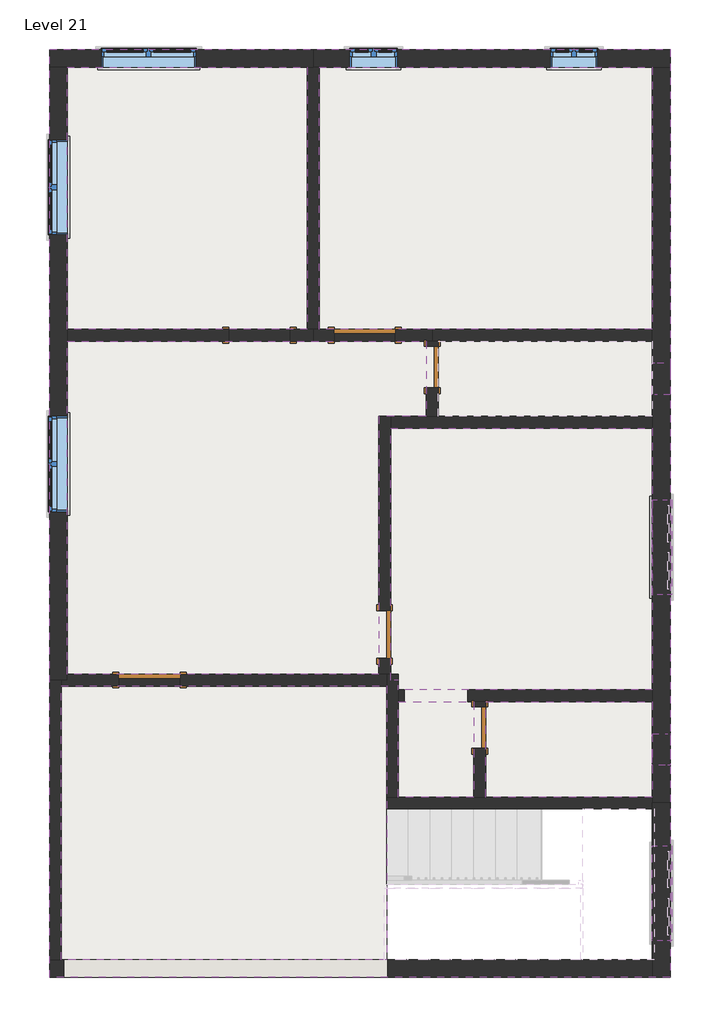
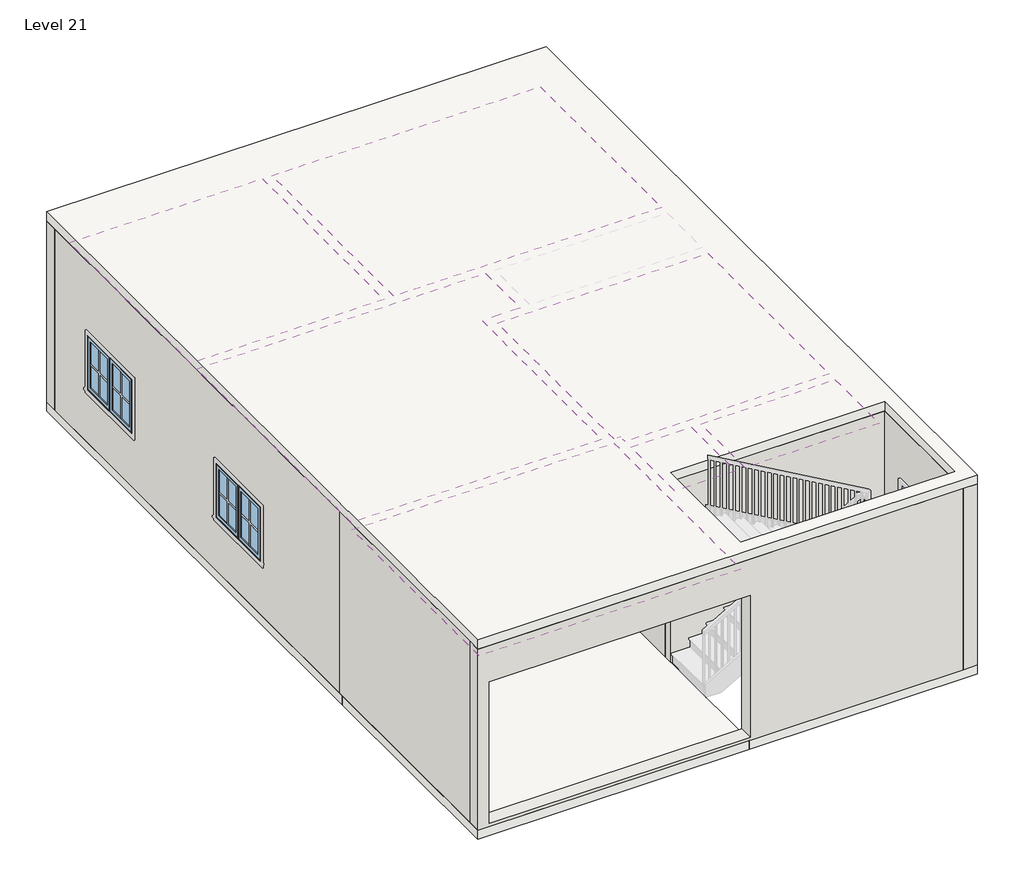
# One storey, part 1 of 2: 27 walls, 13 windows, 7 coverings, 6 doors, 3 slabs.
"""IFC4 building model written with IfcOpenShell, lengths in millimetres."""

from ifc_helpers import new_model, si_unit, frame, origin, place, context, project, spatial, polyline, outline, extrude, faceted_brep, transform, mapped, element, save
from components import door_2908be75, door_9ea4ff49, door_dc34e247, door_b804d09e, fixed_2_415b3208, window_casement_double_3_c417fced, window_casement_double_4_c19c33cb

model = new_model("IFC4")

# Units and contexts
model_context = context("Model", 3, world=origin())
ifc_project = project(units=[si_unit("LENGTHUNIT", "METRE", prefix="MILLI")], contexts=[model_context])

# Site, building, storey
site = spatial("IfcSite", under=ifc_project)
building = spatial("IfcBuilding", under=site)
storey = spatial("IfcBuildingStorey", under=building, Name="Level 21", Elevation=16002.0)

# Coverings
placement = place(None, origin())
element("IfcCovering", 1, ObjectType="2' x 4' ACT System", at=placement, inside=storey, context=model_context, shape_type="SweptSolid", body=[
    extrude(outline(polyline([(-5680.5154463, 2323.8455275), (-5680.5154463, 5678.2330275), (-2607.1154463, 5678.2330275), (-2607.1154463, 2323.8455275), (-5680.5154463, 2323.8455275)])), frame((0.0, 0.0, 18745.2), z_axis=(0.0, 0.0, 1.0), x_axis=(1.0, 0.0, 0.0)), (0.0, 0.0, 1.0), 57.15),
])
element("IfcCovering", 2, ObjectType="2' x 4' ACT System", at=placement, inside=storey, context=model_context, shape_type="SweptSolid", body=[
    extrude(outline(polyline([(-2454.7154463, 2323.8455275), (-2454.7154463, 5678.2330275), (1812.4845537, 5678.2330275), (1812.4845537, 2323.8455275), (-2454.7154463, 2323.8455275)])), frame((0.0, 0.0, 18745.2), z_axis=(0.0, 0.0, 1.0), x_axis=(1.0, 0.0, 0.0)), (0.0, 0.0, 1.0), 57.15),
])
element("IfcCovering", 3, ObjectType="2' x 4' ACT System", at=placement, inside=storey, context=model_context, shape_type="SweptSolid", body=[
    extrude(outline(polyline([(-5680.5154463, -2095.7544725), (-5680.5154463, 2171.4455275), (-1083.1154463, 2171.4455275), (-1083.1154463, 1206.2455275), (-1692.7154463, 1206.2455275), (-1692.7154463, -2095.7544725), (-5680.5154463, -2095.7544725)])), frame((0.0, 0.0, 18745.2), z_axis=(0.0, 0.0, 1.0), x_axis=(1.0, 0.0, 0.0)), (0.0, 0.0, 1.0), 57.15),
])
element("IfcCovering", 4, ObjectType="2' x 4' ACT System", at=placement, inside=storey, context=model_context, shape_type="SweptSolid", body=[
    extrude(outline(polyline([(1812.4845537, 1053.8455275), (1812.4845537, -2298.9544725), (-1438.7154463, -2298.9544725), (-1438.7154463, -2171.9544725), (-1540.3154463, -2171.9544725), (-1540.3154463, 1053.8455275), (1812.4845537, 1053.8455275)])), frame((0.0, 0.0, 18745.2), z_axis=(0.0, 0.0, 1.0), x_axis=(1.0, 0.0, 0.0)), (0.0, 0.0, 1.0), 57.15),
])
element("IfcCovering", 5, ObjectType="2' x 4' ACT System", at=placement, inside=storey, context=model_context, shape_type="SweptSolid", body=[
    extrude(outline(polyline([(1812.4845537, -2451.3544725), (1812.4845537, -3670.5544725), (-321.1154463, -3670.5544725), (-321.1154463, -2451.3544725), (1812.4845537, -2451.3544725)])), frame((0.0, 0.0, 18745.2), z_axis=(0.0, 0.0, 1.0), x_axis=(1.0, 0.0, 0.0)), (0.0, 0.0, 1.0), 57.15),
])
element("IfcCovering", 6, ObjectType="2' x 4' ACT System", at=placement, inside=storey, context=model_context, shape_type="SweptSolid", body=[
    extrude(outline(polyline([(-473.5154463, -2451.3544725), (-473.5154463, -3670.5544725), (-1438.7154463, -3670.5544725), (-1438.7154463, -2451.3544725), (-473.5154463, -2451.3544725)])), frame((0.0, 0.0, 18745.2), z_axis=(0.0, 0.0, 1.0), x_axis=(1.0, 0.0, 0.0)), (0.0, 0.0, 1.0), 57.15),
])
element("IfcCovering", 7, ObjectType="2' x 4' ACT System", at=placement, inside=storey, context=model_context, shape_type="SweptSolid", body=[
    extrude(outline(polyline([(-1591.1154463, -2248.1544725), (-1591.1154463, -5753.3544725), (-5756.7154463, -5753.3544725), (-5756.7154463, -2248.1544725), (-1591.1154463, -2248.1544725)])), frame((0.0, 0.0, 18745.2), z_axis=(0.0, 0.0, 1.0), x_axis=(1.0, 0.0, 0.0)), (0.0, 0.0, 1.0), 57.15),
])

# Doors
door_shape = door_2908be75(model_context)
element("IfcDoor", 8, ObjectType="Single-Flush : 1' 9\"", at=placement, inside=storey, context=model_context, shape_type="MappedRepresentation", body=[
    mapped(door_shape, transform((-397.3154463, -2781.5544725, 16002.0), x_axis=(0.0, 1.0, 0.0), y_axis=(-1.0, 0.0, 0.0), z_axis=(0.0, 0.0, 1.0))),
])
element("IfcDoor", 9, ObjectType="Single-Flush : 1' 9\"", at=placement, inside=storey, context=model_context, shape_type="MappedRepresentation", body=[
    mapped(door_shape, transform((-1006.9154463, 1841.2455275, 16002.0), x_axis=(0.0, 1.0, 0.0), y_axis=(-1.0, 0.0, 0.0), z_axis=(0.0, 0.0, 1.0))),
])
door_2_shape = door_9ea4ff49(model_context)
element("IfcDoor", 10, ObjectType="Single-Flush : 2'0\"", at=placement, inside=storey, context=model_context, shape_type="MappedRepresentation", body=[
    mapped(door_2_shape, transform((-1616.5154463, -1587.7544725, 16002.0), x_axis=(0.0, -1.0, 0.0), y_axis=(1.0, 0.0, 0.0), z_axis=(0.0, 0.0, 1.0))),
])
door_3_shape = door_dc34e247(model_context)
element("IfcDoor", 11, ObjectType="Single-Flush : 2'7\"", at=placement, inside=storey, context=model_context, shape_type="MappedRepresentation", body=[
    mapped(door_3_shape, transform((-4626.4154463, -2171.9544725, 16002.0), x_axis=(-1.0, 0.0, 0.0), y_axis=(0.0, -1.0, 0.0), z_axis=(0.0, 0.0, 1.0))),
])
element("IfcDoor", 12, ObjectType="Single-Flush : 2'7\"", at=placement, inside=storey, context=model_context, shape_type="MappedRepresentation", body=[
    mapped(door_3_shape, transform((-1870.5154463, 2247.6455275, 16002.0), x_axis=(-1.0, 0.0, 0.0), y_axis=(0.0, -1.0, 0.0), z_axis=(0.0, 0.0, 1.0))),
])
door_4_shape = door_b804d09e(model_context)
element("IfcDoor", 13, ObjectType="Single-Flush : 2'7\"", at=placement, inside=storey, context=model_context, shape_type="MappedRepresentation", body=[
    mapped(door_4_shape, transform((-3216.7154463, 2247.6455275, 16002.0), x_axis=(1.0, 0.0, 0.0), y_axis=(0.0, 1.0, 0.0), z_axis=(0.0, 0.0, 1.0))),
])

# Slabs
element("IfcSlab", 14, ObjectType="Generic - 6\"", at=placement, inside=storey, context=model_context, shape_type="SweptSolid", body=[
    extrude(outline(polyline([(-5909.1154463, -2248.1544725), (-5909.1154463, 5906.8330275), (2041.0845537, 5906.8330275), (2041.0845537, -5981.9544725), (-1591.1154463, -5981.9544725), (-1591.1154463, -5753.3544725), (1812.4845537, -5753.3544725), (1812.4845537, -3822.9544725), (-1591.1154463, -3822.9544725), (-1591.1154463, -2248.1544725), (-5756.7154463, -2248.1544725), (-5909.1154463, -2248.1544725)])), frame((0.0, 0.0, 15849.6), z_axis=(0.0, 0.0, 1.0), x_axis=(1.0, 0.0, 0.0)), (0.0, 0.0, 1.0), 152.4),
])
element("IfcSlab", 15, ObjectType="Generic - 6\"", at=placement, inside=storey, context=model_context, shape_type="SweptSolid", body=[
    extrude(outline(polyline([(-1591.1154463, -2248.1544725), (-1591.1154463, -5981.9544725), (-5909.1154463, -5981.9544725), (-5909.1154463, -2248.1544725), (-1591.1154463, -2248.1544725)])), frame((0.0, 0.0, 15849.6), z_axis=(0.0, 0.0, 1.0), x_axis=(1.0, 0.0, 0.0)), (0.0, 0.0, 1.0), 152.4),
])
element("IfcSlab", 16, ObjectType="Generic - 6\"", at=placement, inside=storey, context=model_context, shape_type="SweptSolid", body=[
    extrude(outline(polyline([(2041.0845537, 5906.8330275), (2041.0845537, -5981.9544725), (-5909.1154463, -5981.9544725), (-5909.1154463, 5906.8330275), (2041.0845537, 5906.8330275)]), holes=[polyline([(1812.4845537, -3822.9544725), (-1591.1154463, -3822.9544725), (-1591.1154463, -5753.3544725), (1812.4845537, -5753.3544725), (1812.4845537, -3822.9544725)])]), frame((0.0, 0.0, 19050.0), z_axis=(0.0, 0.0, 1.0), x_axis=(1.0, 0.0, 0.0)), (0.0, 0.0, 1.0), 152.4),
])

# Walls
element("IfcWall", 17, ObjectType="Generic - 6\"", at=placement, inside=storey, context=model_context, shape_type="Brep", body=[
    faceted_brep([(-5909.1154463, -2171.9544725, 16002.0), (-5909.1154463, -5753.3544725, 16002.0), (-5909.1154463, -5753.3544725, 19050.0), (-5909.1154463, -2171.9544725, 19050.0), (-5756.7154463, -2171.9544725, 16002.0), (-5756.7154463, -2171.9544725, 19050.0), (-5756.7154463, -2248.1544725, 19050.0), (-5756.7154463, -5753.3544725, 19050.0), (-5756.7154463, -5753.3544725, 16002.0), (-5756.7154463, -2248.1544725, 16002.0)], [[[0, 1, 2, 3]], [[4, 5, 6, 7, 8, 9]], [[1, 0, 4, 9, 8]], [[3, 2, 7, 6, 5]], [[0, 3, 5, 4]], [[2, 1, 8, 7]]]),
])
element("IfcWall", 18, ObjectType="Generic - 6\"", at=placement, inside=storey, context=model_context, shape_type="Brep", body=[
    faceted_brep([(1812.4845537, -3670.5544725, 16002.0), (-321.1154463, -3670.5544725, 16002.0), (-473.5154463, -3670.5544725, 16002.0), (-1438.7154463, -3670.5544725, 16002.0), (-1591.1154463, -3670.5544725, 16002.0), (-1591.1154463, -3670.5544725, 19050.0), (-1438.7154463, -3670.5544725, 19050.0), (-473.5154463, -3670.5544725, 19050.0), (-321.1154463, -3670.5544725, 19050.0), (1812.4845537, -3670.5544725, 19050.0), (1812.4845537, -3822.9544725, 16002.0), (1812.4845537, -3822.9544725, 19050.0), (-1591.1154463, -3822.9544725, 19050.0), (-1591.1154463, -3822.9544725, 16002.0), (1812.4845537, -3746.7544725, 16002.0), (1812.4845537, -3746.7544725, 19050.0)], [[[0, 1, 2, 3, 4, 5, 6, 7, 8, 9]], [[10, 11, 12, 13]], [[4, 3, 2, 1, 0, 14, 10, 13]], [[9, 8, 7, 6, 5, 12, 11, 15]], [[5, 4, 13, 12]], [[0, 9, 15, 11, 10, 14]]]),
])
element("IfcWall", 19, ObjectType="Generic - 6\"", at=placement, inside=storey, context=model_context, shape_type="Brep", body=[
    faceted_brep([(-1438.7154463, -3670.5544725, 16002.0), (-1438.7154463, -2451.3544725, 16002.0), (-1438.7154463, -2298.9544725, 16002.0), (-1438.7154463, -2095.7544725, 16002.0), (-1438.7154463, -2095.7544725, 19050.0), (-1438.7154463, -2298.9544725, 19050.0), (-1438.7154463, -2451.3544725, 19050.0), (-1438.7154463, -3670.5544725, 19050.0), (-1591.1154463, -3670.5544725, 16002.0), (-1591.1154463, -3670.5544725, 19050.0), (-1591.1154463, -2248.1544725, 19050.0), (-1591.1154463, -2171.9544725, 19050.0), (-1591.1154463, -2095.7544725, 19050.0), (-1591.1154463, -2095.7544725, 16002.0), (-1591.1154463, -2171.9544725, 16002.0), (-1591.1154463, -2248.1544725, 16002.0), (-1540.3154463, -2095.7544725, 16002.0), (-1540.3154463, -2095.7544725, 19050.0)], [[[0, 1, 2, 3, 4, 5, 6, 7]], [[8, 9, 10, 11, 12, 13, 14, 15]], [[3, 2, 1, 0, 8, 15, 14, 13, 16]], [[7, 6, 5, 4, 17, 12, 11, 10, 9]], [[0, 7, 9, 8]], [[4, 3, 16, 13, 12, 17]]]),
])
element("IfcWall", 20, ObjectType="Generic - 6\"", at=placement, inside=storey, context=model_context, shape_type="Brep", body=[
    faceted_brep([(-5020.1154463, -2095.7544725, 18135.6), (-5020.1154463, -2095.7544725, 16002.0), (-5680.5154463, -2095.7544725, 16002.0), (-5680.5154463, -2095.7544725, 19050.0), (-1692.7154463, -2095.7544725, 19050.0), (-1591.1154463, -2095.7544725, 19050.0), (-1591.1154463, -2095.7544725, 16002.0), (-1692.7154463, -2095.7544725, 16002.0), (-4232.7154463, -2095.7544725, 16002.0), (-4232.7154463, -2095.7544725, 18135.6), (-5756.7154463, -2248.1544725, 16002.0), (-5020.1154463, -2248.1544725, 16002.0), (-5020.1154463, -2248.1544725, 18135.6), (-4232.7154463, -2248.1544725, 18135.6), (-4232.7154463, -2248.1544725, 16002.0), (-1591.1154463, -2248.1544725, 16002.0), (-1591.1154463, -2248.1544725, 19050.0), (-5756.7154463, -2248.1544725, 19050.0), (-5756.7154463, -2171.9544725, 16002.0), (-5680.5154463, -2171.9544725, 16002.0), (-5680.5154463, -2171.9544725, 19050.0), (-5756.7154463, -2171.9544725, 19050.0)], [[[0, 1, 2, 3, 4, 5, 6, 7, 8, 9]], [[10, 11, 12, 13, 14, 15, 16, 17]], [[2, 1, 11, 10, 18, 19]], [[8, 7, 6, 15, 14]], [[5, 4, 3, 20, 21, 17, 16]], [[3, 2, 19, 20]], [[19, 18, 21, 20]], [[18, 10, 17, 21]], [[6, 5, 16, 15]], [[12, 11, 1, 0]], [[13, 12, 0, 9]], [[14, 13, 9, 8]]]),
])
element("IfcWall", 21, ObjectType="Generic - 6\"", at=placement, inside=storey, context=model_context, shape_type="Brep", body=[
    faceted_brep([(1812.4845537, -2451.3544725, 16002.0), (1812.4845537, -2451.3544725, 19050.0), (-321.1154463, -2451.3544725, 19050.0), (-473.5154463, -2451.3544725, 19050.0), (-1438.7154463, -2451.3544725, 19050.0), (-1438.7154463, -2451.3544725, 16002.0), (-1367.0206652, -2451.3544725, 16002.0), (-1367.0206652, -2451.3544725, 18440.4), (-547.4818767, -2451.3544725, 18440.4), (-547.4818767, -2451.3544725, 16002.0), (-473.5154463, -2451.3544725, 16002.0), (-321.1154463, -2451.3544725, 16002.0), (1812.4845537, -2298.9544725, 19050.0), (1812.4845537, -2298.9544725, 16002.0), (-547.4818767, -2298.9544725, 16002.0), (-547.4818767, -2298.9544725, 18440.4), (-1367.0206652, -2298.9544725, 18440.4), (-1367.0206652, -2298.9544725, 16002.0), (-1438.7154463, -2298.9544725, 16002.0), (-1438.7154463, -2298.9544725, 19050.0)], [[[0, 1, 2, 3, 4, 5, 6, 7, 8, 9, 10, 11]], [[12, 13, 14, 15, 16, 17, 18, 19]], [[5, 18, 17, 6]], [[13, 0, 11, 10, 9, 14]], [[4, 3, 2, 1, 12, 19]], [[1, 0, 13, 12]], [[5, 4, 19, 18]], [[7, 16, 15, 8]], [[16, 7, 6, 17]], [[8, 15, 14, 9]]]),
])
element("IfcWall", 22, ObjectType="Generic - 6\"", at=placement, inside=storey, context=model_context, shape_type="SweptSolid", body=[
    extrude(outline(polyline([(-2451.3544725, 16002.0), (-2514.8544725, 16002.0), (-2514.8544725, 18135.6), (-3048.2544725, 18135.6), (-3048.2544725, 16002.0), (-3670.5544725, 16002.0), (-3670.5544725, 19050.0), (-2451.3544725, 19050.0), (-2451.3544725, 16002.0)])), frame((-473.5154463, 0.0, 0.0), z_axis=(1.0, 0.0, 0.0), x_axis=(0.0, 1.0, 0.0)), (0.0, 0.0, 1.0), 152.4),
])
element("IfcWall", 23, ObjectType="Generic - 6\"", at=placement, inside=storey, context=model_context, shape_type="Brep", body=[
    faceted_brep([(-1540.3154463, -2095.7544725, 16002.0), (-1540.3154463, -1892.5544725, 16002.0), (-1540.3154463, -1892.5544725, 18135.6), (-1540.3154463, -1282.9544725, 18135.6), (-1540.3154463, -1282.9544725, 16002.0), (-1540.3154463, 1053.8455275, 16002.0), (-1540.3154463, 1206.2455275, 16002.0), (-1540.3154463, 1206.2455275, 19050.0), (-1540.3154463, 1053.8455275, 19050.0), (-1540.3154463, -2095.7544725, 19050.0), (-1692.7154463, -1892.5544725, 18135.6), (-1692.7154463, -1892.5544725, 16002.0), (-1692.7154463, -2095.7544725, 16002.0), (-1692.7154463, -2095.7544725, 19050.0), (-1692.7154463, 1206.2455275, 19050.0), (-1692.7154463, 1206.2455275, 16002.0), (-1692.7154463, -1282.9544725, 16002.0), (-1692.7154463, -1282.9544725, 18135.6), (-1591.1154463, -2095.7544725, 16002.0), (-1591.1154463, -2095.7544725, 19050.0)], [[[0, 1, 2, 3, 4, 5, 6, 7, 8, 9]], [[10, 11, 12, 13, 14, 15, 16, 17]], [[16, 15, 6, 5, 4]], [[12, 11, 1, 0, 18]], [[9, 8, 7, 14, 13, 19]], [[0, 9, 19, 13, 12, 18]], [[7, 6, 15, 14]], [[2, 1, 11, 10]], [[3, 2, 10, 17]], [[4, 3, 17, 16]]]),
])
element("IfcWall", 24, ObjectType="Generic - 6\"", at=placement, inside=storey, context=model_context, shape_type="Brep", body=[
    faceted_brep([(-1540.3154463, 1053.8455275, 16002.0), (1812.4845537, 1053.8455275, 16002.0), (1812.4845537, 1053.8455275, 19050.0), (-1540.3154463, 1053.8455275, 19050.0), (-1540.3154463, 1206.2455275, 16002.0), (-1540.3154463, 1206.2455275, 19050.0), (-1083.1154463, 1206.2455275, 19050.0), (-930.7154463, 1206.2455275, 19050.0), (1812.4845537, 1206.2455275, 19050.0), (1812.4845537, 1206.2455275, 16002.0), (-930.7154463, 1206.2455275, 16002.0), (-1083.1154463, 1206.2455275, 16002.0)], [[[0, 1, 2, 3]], [[4, 5, 6, 7, 8, 9, 10, 11]], [[1, 0, 4, 11, 10, 9]], [[3, 2, 8, 7, 6, 5]], [[0, 3, 5, 4]], [[2, 1, 9, 8]]]),
])
element("IfcWall", 25, ObjectType="Generic - 6\"", at=placement, inside=storey, context=model_context, shape_type="Brep", body=[
    faceted_brep([(-930.7154463, 2107.9455275, 18135.6), (-930.7154463, 2107.9455275, 16002.0), (-930.7154463, 2171.4455275, 16002.0), (-930.7154463, 2171.4455275, 19050.0), (-930.7154463, 1206.2455275, 19050.0), (-930.7154463, 1206.2455275, 16002.0), (-930.7154463, 1574.5455275, 16002.0), (-930.7154463, 1574.5455275, 18135.6), (-1083.1154463, 2171.4455275, 16002.0), (-1083.1154463, 2107.9455275, 16002.0), (-1083.1154463, 2107.9455275, 18135.6), (-1083.1154463, 1574.5455275, 18135.6), (-1083.1154463, 1574.5455275, 16002.0), (-1083.1154463, 1206.2455275, 16002.0), (-1083.1154463, 1206.2455275, 19050.0), (-1083.1154463, 2171.4455275, 19050.0), (-1006.9154463, 2171.4455275, 16002.0), (-1006.9154463, 2171.4455275, 19050.0)], [[[0, 1, 2, 3, 4, 5, 6, 7]], [[8, 9, 10, 11, 12, 13, 14, 15]], [[6, 5, 13, 12]], [[2, 1, 9, 8, 16]], [[4, 3, 17, 15, 14]], [[5, 4, 14, 13]], [[10, 9, 1, 0]], [[11, 10, 0, 7]], [[12, 11, 7, 6]], [[3, 2, 16, 8, 15, 17]]]),
])
element("IfcWall", 26, ObjectType="Generic - 6\"", at=placement, inside=storey, context=model_context, shape_type="Brep", body=[
    faceted_brep([(1812.4845537, 2323.8455275, 16002.0), (-1006.9154463, 2323.8455275, 16002.0), (-1006.9154463, 2323.8455275, 19050.0), (1812.4845537, 2323.8455275, 19050.0), (1812.4845537, 2171.4455275, 16002.0), (1812.4845537, 2171.4455275, 19050.0), (-930.7154463, 2171.4455275, 19050.0), (-1006.9154463, 2171.4455275, 19050.0), (-1006.9154463, 2171.4455275, 16002.0), (-930.7154463, 2171.4455275, 16002.0)], [[[0, 1, 2, 3]], [[4, 5, 6, 7, 8, 9]], [[1, 0, 4, 9, 8]], [[2, 1, 8, 7]], [[3, 2, 7, 6, 5]], [[0, 3, 5, 4]]]),
])
element("IfcWall", 27, ObjectType="Generic - 6\"", at=placement, inside=storey, context=model_context, shape_type="Brep", body=[
    faceted_brep([(-2607.1154463, 5678.2330275, 16002.0), (-2607.1154463, 2323.8455275, 16002.0), (-2607.1154463, 2323.8455275, 19050.0), (-2607.1154463, 5678.2330275, 19050.0), (-2454.7154463, 5678.2330275, 16002.0), (-2454.7154463, 5678.2330275, 19050.0), (-2454.7154463, 2323.8455275, 19050.0), (-2454.7154463, 2323.8455275, 16002.0), (-2530.9154463, 5678.2330275, 16002.0), (-2530.9154463, 2323.8455275, 16002.0), (-2530.9154463, 2323.8455275, 19050.0), (-2530.9154463, 5678.2330275, 19050.0)], [[[0, 1, 2, 3]], [[4, 5, 6, 7]], [[1, 0, 8, 4, 7, 9]], [[3, 2, 10, 6, 5, 11]], [[0, 3, 11, 5, 4, 8]], [[2, 1, 9, 7, 6, 10]]]),
])
element("IfcWall", 28, ObjectType="Generic - 6\"", at=placement, inside=storey, context=model_context, shape_type="Brep", body=[
    faceted_brep([(-2530.9154463, 2323.8455275, 16002.0), (-2607.1154463, 2323.8455275, 16002.0), (-2823.0154463, 2323.8455275, 16002.0), (-2823.0154463, 2323.8455275, 18135.6), (-3610.4154463, 2323.8455275, 18135.6), (-3610.4154463, 2323.8455275, 16002.0), (-5680.5154463, 2323.8455275, 16002.0), (-5680.5154463, 2323.8455275, 19050.0), (-2607.1154463, 2323.8455275, 19050.0), (-2530.9154463, 2323.8455275, 19050.0), (-2823.0154463, 2171.4455275, 18135.6), (-2823.0154463, 2171.4455275, 16002.0), (-2530.9154463, 2171.4455275, 16002.0), (-2530.9154463, 2171.4455275, 19050.0), (-5680.5154463, 2171.4455275, 19050.0), (-5680.5154463, 2171.4455275, 16002.0), (-3610.4154463, 2171.4455275, 16002.0), (-3610.4154463, 2171.4455275, 18135.6)], [[[0, 1, 2, 3, 4, 5, 6, 7, 8, 9]], [[10, 11, 12, 13, 14, 15, 16, 17]], [[16, 15, 6, 5]], [[12, 11, 2, 1, 0]], [[9, 8, 7, 14, 13]], [[0, 9, 13, 12]], [[7, 6, 15, 14]], [[5, 4, 17, 16]], [[4, 3, 10, 17]], [[3, 2, 11, 10]]]),
])
element("IfcWall", 29, ObjectType="Generic - 6\"", at=placement, inside=storey, context=model_context, shape_type="Brep", body=[
    faceted_brep([(-2264.2154463, 2323.8455275, 18135.6), (-2264.2154463, 2323.8455275, 16002.0), (-2454.7154463, 2323.8455275, 16002.0), (-2530.9154463, 2323.8455275, 16002.0), (-2530.9154463, 2323.8455275, 19050.0), (-2454.7154463, 2323.8455275, 19050.0), (-1006.9154463, 2323.8455275, 19050.0), (-1006.9154463, 2323.8455275, 16002.0), (-1476.8154463, 2323.8455275, 16002.0), (-1476.8154463, 2323.8455275, 18135.6), (-2530.9154463, 2171.4455275, 16002.0), (-2264.2154463, 2171.4455275, 16002.0), (-2264.2154463, 2171.4455275, 18135.6), (-1476.8154463, 2171.4455275, 18135.6), (-1476.8154463, 2171.4455275, 16002.0), (-1083.1154463, 2171.4455275, 16002.0), (-1006.9154463, 2171.4455275, 16002.0), (-1006.9154463, 2171.4455275, 19050.0), (-1083.1154463, 2171.4455275, 19050.0), (-2530.9154463, 2171.4455275, 19050.0)], [[[0, 1, 2, 3, 4, 5, 6, 7, 8, 9]], [[10, 11, 12, 13, 14, 15, 16, 17, 18, 19]], [[8, 7, 16, 15, 14]], [[3, 2, 1, 11, 10]], [[4, 3, 10, 19]], [[6, 5, 4, 19, 18, 17]], [[7, 6, 17, 16]], [[14, 13, 9, 8]], [[13, 12, 0, 9]], [[12, 11, 1, 0]]]),
])
element("IfcWall", 30, ObjectType="Generic - 6\"", at=placement, inside=storey, context=model_context, shape_type="SweptSolid", body=[
    extrude(outline(polyline([(-5680.5154463, -2095.7544725), (-1692.7154463, -2095.7544725), (-1692.7154463, -2171.9544725), (-1591.1154463, -2171.9544725), (-1591.1154463, -2248.1544725), (-5756.7154463, -2248.1544725), (-5756.7154463, -2171.9544725), (-5680.5154463, -2171.9544725), (-5680.5154463, -2095.7544725)])), frame((0.0, 0.0, 16002.0), z_axis=(0.0, 0.0, 1.0), x_axis=(1.0, 0.0, 0.0)), (0.0, 0.0, 1.0), 3048.0),
])
element("IfcWall", 31, ObjectType="Generic - 6\"", at=placement, inside=storey, context=model_context, shape_type="Brep", body=[
    faceted_brep([(-2607.1154463, 5678.2330275, 16002.0), (-2607.1154463, 2323.8455275, 16002.0), (-2607.1154463, 2323.8455275, 19050.0), (-2607.1154463, 5678.2330275, 19050.0), (-2454.7154463, 5678.2330275, 16002.0), (-2454.7154463, 5678.2330275, 19050.0), (-2454.7154463, 2323.8455275, 19050.0), (-2454.7154463, 2323.8455275, 16002.0), (-2530.9154463, 5678.2330275, 16002.0), (-2530.9154463, 2323.8455275, 16002.0), (-2530.9154463, 2323.8455275, 19050.0), (-2530.9154463, 5678.2330275, 19050.0)], [[[0, 1, 2, 3]], [[4, 5, 6, 7]], [[1, 0, 8, 4, 7, 9]], [[3, 2, 10, 6, 5, 11]], [[0, 3, 11, 5, 4, 8]], [[2, 1, 9, 7, 6, 10]]]),
])
element("IfcWall", 32, ObjectType="Generic - 6\"", at=placement, inside=storey, context=model_context, shape_type="Brep", body=[
    faceted_brep([(-2530.9154463, 2323.8455275, 16002.0), (-2607.1154463, 2323.8455275, 16002.0), (-5680.5154463, 2323.8455275, 16002.0), (-5680.5154463, 2323.8455275, 19050.0), (-2607.1154463, 2323.8455275, 19050.0), (-2530.9154463, 2323.8455275, 19050.0), (-2530.9154463, 2171.4455275, 16002.0), (-2530.9154463, 2171.4455275, 19050.0), (-5680.5154463, 2171.4455275, 19050.0), (-5680.5154463, 2171.4455275, 16002.0)], [[[0, 1, 2, 3, 4, 5]], [[6, 7, 8, 9]], [[2, 1, 0, 6, 9]], [[5, 4, 3, 8, 7]], [[0, 5, 7, 6]], [[3, 2, 9, 8]]]),
])
element("IfcWall", 33, ObjectType="Generic - 6\"", at=placement, inside=storey, context=model_context, shape_type="Brep", body=[
    faceted_brep([(-1006.9154463, 2323.8455275, 16002.0), (-2454.7154463, 2323.8455275, 16002.0), (-2530.9154463, 2323.8455275, 16002.0), (-2530.9154463, 2323.8455275, 19050.0), (-2454.7154463, 2323.8455275, 19050.0), (-1006.9154463, 2323.8455275, 19050.0), (-1006.9154463, 2171.4455275, 16002.0), (-1006.9154463, 2171.4455275, 19050.0), (-1083.1154463, 2171.4455275, 19050.0), (-2530.9154463, 2171.4455275, 19050.0), (-2530.9154463, 2171.4455275, 16002.0), (-1083.1154463, 2171.4455275, 16002.0)], [[[0, 1, 2, 3, 4, 5]], [[6, 7, 8, 9, 10, 11]], [[2, 1, 0, 6, 11, 10]], [[3, 2, 10, 9]], [[5, 4, 3, 9, 8, 7]], [[0, 5, 7, 6]]]),
])
element("IfcWall", 34, ObjectType="Generic - 9\"", at=placement, inside=storey, context=model_context, shape_type="Brep", body=[
    faceted_brep([(-5909.1154463, 5678.2330275, 16002.0), (-5680.5154463, 5678.2330275, 16002.0), (-2607.1154463, 5678.2330275, 16002.0), (-2530.9154463, 5678.2330275, 16002.0), (-2530.9154463, 5678.2330275, 19050.0), (-2607.1154463, 5678.2330275, 19050.0), (-5680.5154463, 5678.2330275, 19050.0), (-5909.1154463, 5678.2330275, 19050.0), (-4029.5154463, 5678.2330275, 17830.8), (-4029.5154463, 5678.2330275, 16916.4), (-5248.7154463, 5678.2330275, 16916.4), (-5248.7154463, 5678.2330275, 17830.8), (-5909.1154463, 5906.8330275, 16002.0), (-5909.1154463, 5906.8330275, 19050.0), (-2530.9154463, 5906.8330275, 19050.0), (-2530.9154463, 5906.8330275, 16002.0), (-4029.5154463, 5906.8330275, 17830.8), (-5248.7154463, 5906.8330275, 17830.8), (-5248.7154463, 5906.8330275, 16916.4), (-4029.5154463, 5906.8330275, 16916.4)], [[[0, 1, 2, 3, 4, 5, 6, 7], [8, 9, 10, 11]], [[12, 13, 14, 15], [16, 17, 18, 19]], [[3, 2, 1, 0, 12, 15]], [[4, 3, 15, 14]], [[7, 6, 5, 4, 14, 13]], [[0, 7, 13, 12]], [[9, 8, 16, 19]], [[10, 9, 19, 18]], [[11, 10, 18, 17]], [[8, 11, 17, 16]]]),
])
element("IfcWall", 35, ObjectType="Generic - 9\"", at=placement, inside=storey, context=model_context, shape_type="Brep", body=[
    faceted_brep([(1812.4845537, 5678.2330275, 16002.0), (1812.4845537, 2323.8455275, 16002.0), (1812.4845537, 2171.4455275, 16002.0), (1812.4845537, 1206.2455275, 16002.0), (1812.4845537, 1053.8455275, 16002.0), (1812.4845537, -2298.9544725, 16002.0), (1812.4845537, -2451.3544725, 16002.0), (1812.4845537, -3670.5544725, 16002.0), (1812.4845537, -3746.7544725, 16002.0), (1812.4845537, -3746.7544725, 19050.0), (1812.4845537, -3670.5544725, 19050.0), (1812.4845537, -2451.3544725, 19050.0), (1812.4845537, -2298.9544725, 19050.0), (1812.4845537, 1053.8455275, 19050.0), (1812.4845537, 1206.2455275, 19050.0), (1812.4845537, 2171.4455275, 19050.0), (1812.4845537, 2323.8455275, 19050.0), (1812.4845537, 5678.2330275, 19050.0), (1812.4845537, -1079.7544725, 18135.6), (1812.4845537, -1079.7544725, 17221.2), (1812.4845537, 139.4455275, 17221.2), (1812.4845537, 139.4455275, 18135.6), (1812.4845537, -3264.1544725, 18440.4), (1812.4845537, -3264.1544725, 17830.8), (1812.4845537, -2857.7544725, 17830.8), (1812.4845537, -2857.7544725, 18440.4), (1812.4845537, 1892.0455275, 18440.4), (1812.4845537, 1485.6455275, 18440.4), (1812.4845537, 1485.6455275, 17830.8), (1812.4845537, 1892.0455275, 17830.8), (2041.0845537, 5678.2330275, 16002.0), (2041.0845537, 5678.2330275, 19050.0), (2041.0845537, -3746.7544725, 19050.0), (2041.0845537, -3746.7544725, 16002.0), (2041.0845537, -1079.7544725, 18135.6), (2041.0845537, 139.4455275, 18135.6), (2041.0845537, 139.4455275, 17221.2), (2041.0845537, -1079.7544725, 17221.2), (2041.0845537, -3264.1544725, 18440.4), (2041.0845537, -2857.7544725, 18440.4), (2041.0845537, -2857.7544725, 17830.8), (2041.0845537, -3264.1544725, 17830.8), (2041.0845537, 1892.0455275, 18440.4), (2041.0845537, 1892.0455275, 17830.8), (2041.0845537, 1485.6455275, 17830.8), (2041.0845537, 1485.6455275, 18440.4)], [[[0, 1, 2, 3, 4, 5, 6, 7, 8, 9, 10, 11, 12, 13, 14, 15, 16, 17], [18, 19, 20, 21], [22, 23, 24, 25], [26, 27, 28, 29]], [[30, 31, 32, 33], [34, 35, 36, 37], [38, 39, 40, 41], [42, 43, 44, 45]], [[8, 7, 6, 5, 4, 3, 2, 1, 0, 30, 33]], [[9, 8, 33, 32]], [[17, 16, 15, 14, 13, 12, 11, 10, 9, 32, 31]], [[0, 17, 31, 30]], [[19, 18, 34, 37]], [[20, 19, 37, 36]], [[21, 20, 36, 35]], [[18, 21, 35, 34]], [[23, 22, 38, 41]], [[24, 23, 41, 40]], [[25, 24, 40, 39]], [[22, 25, 39, 38]], [[43, 42, 26, 29]], [[44, 43, 29, 28]], [[45, 44, 28, 27]], [[42, 45, 27, 26]]]),
])
element("IfcWall", 36, ObjectType="Generic - 9\"", at=placement, inside=storey, context=model_context, shape_type="Brep", body=[
    faceted_brep([(1812.4845537, -5753.3544725, 16002.0), (-5756.7154463, -5753.3544725, 16002.0), (-5909.1154463, -5753.3544725, 16002.0), (-5909.1154463, -5753.3544725, 19050.0), (-5756.7154463, -5753.3544725, 19050.0), (1812.4845537, -5753.3544725, 19050.0), (-1576.8982041, -5753.3544725, 18440.4), (-5729.1673724, -5753.3544725, 18440.4), (-5729.1673724, -5753.3544725, 16052.8), (-1576.8982041, -5753.3544725, 16052.8), (-5909.1154463, -5981.9544725, 16002.0), (1812.4845537, -5981.9544725, 16002.0), (1812.4845537, -5981.9544725, 19050.0), (-5909.1154463, -5981.9544725, 19050.0), (-5729.1673724, -5981.9544725, 18440.4), (-1576.8982041, -5981.9544725, 18440.4), (-1576.8982041, -5981.9544725, 16052.8), (-5729.1673724, -5981.9544725, 16052.8)], [[[0, 1, 2, 3, 4, 5], [6, 7, 8, 9]], [[10, 11, 12, 13], [14, 15, 16, 17]], [[2, 1, 0, 11, 10]], [[5, 4, 3, 13, 12]], [[0, 5, 12, 11]], [[6, 15, 14, 7]], [[8, 17, 16, 9]], [[15, 6, 9, 16]], [[7, 14, 17, 8]], [[3, 2, 10, 13]]]),
])
element("IfcWall", 37, ObjectType="Generic - 9\"", at=placement, inside=storey, context=model_context, shape_type="Brep", body=[
    faceted_brep([(-5909.1154463, 5678.2330275, 16002.0), (-5909.1154463, -2171.9544725, 16002.0), (-5909.1154463, -2171.9544725, 19050.0), (-5909.1154463, 5678.2330275, 19050.0), (-5909.1154463, 4751.1330275, 17830.8), (-5909.1154463, 3531.9330275, 17830.8), (-5909.1154463, 3531.9330275, 16916.4), (-5909.1154463, 4751.1330275, 16916.4), (-5909.1154463, 1206.2455275, 17830.8), (-5909.1154463, -12.9544725, 17830.8), (-5909.1154463, -12.9544725, 16916.4), (-5909.1154463, 1206.2455275, 16916.4), (-5680.5154463, 5678.2330275, 16002.0), (-5680.5154463, 5678.2330275, 19050.0), (-5680.5154463, 2323.8455275, 19050.0), (-5680.5154463, 2171.4455275, 19050.0), (-5680.5154463, -2095.7544725, 19050.0), (-5680.5154463, -2171.9544725, 19050.0), (-5680.5154463, -2171.9544725, 16002.0), (-5680.5154463, -2095.7544725, 16002.0), (-5680.5154463, 2171.4455275, 16002.0), (-5680.5154463, 2323.8455275, 16002.0), (-5680.5154463, 4751.1330275, 17830.8), (-5680.5154463, 4751.1330275, 16916.4), (-5680.5154463, 3531.9330275, 16916.4), (-5680.5154463, 3531.9330275, 17830.8), (-5680.5154463, 1206.2455275, 17830.8), (-5680.5154463, 1206.2455275, 16916.4), (-5680.5154463, -12.9544725, 16916.4), (-5680.5154463, -12.9544725, 17830.8), (-5756.7154463, -2171.9544725, 16002.0), (-5756.7154463, -2171.9544725, 19050.0)], [[[0, 1, 2, 3], [4, 5, 6, 7], [8, 9, 10, 11]], [[12, 13, 14, 15, 16, 17, 18, 19, 20, 21], [22, 23, 24, 25], [26, 27, 28, 29]], [[1, 0, 12, 21, 20, 19, 18, 30]], [[2, 1, 30, 18, 17, 31]], [[3, 2, 31, 17, 16, 15, 14, 13]], [[0, 3, 13, 12]], [[23, 22, 4, 7]], [[24, 23, 7, 6]], [[25, 24, 6, 5]], [[22, 25, 5, 4]], [[27, 26, 8, 11]], [[28, 27, 11, 10]], [[29, 28, 10, 9]], [[26, 29, 9, 8]]]),
])
element("IfcWall", 38, ObjectType="Generic - 9\"", at=placement, inside=storey, context=model_context, shape_type="Brep", body=[
    faceted_brep([(-2530.9154463, 5678.2330275, 16002.0), (-2454.7154463, 5678.2330275, 16002.0), (1812.4845537, 5678.2330275, 16002.0), (2041.0845537, 5678.2330275, 16002.0), (2041.0845537, 5678.2330275, 19050.0), (1812.4845537, 5678.2330275, 19050.0), (-2454.7154463, 5678.2330275, 19050.0), (-2530.9154463, 5678.2330275, 19050.0), (-1451.4154463, 5678.2330275, 17830.8), (-1451.4154463, 5678.2330275, 16916.4), (-2061.0154463, 5678.2330275, 16916.4), (-2061.0154463, 5678.2330275, 17830.8), (1113.9845537, 5678.2330275, 17830.8), (1113.9845537, 5678.2330275, 16916.4), (504.3845537, 5678.2330275, 16916.4), (504.3845537, 5678.2330275, 17830.8), (-2530.9154463, 5906.8330275, 16002.0), (-2530.9154463, 5906.8330275, 19050.0), (2041.0845537, 5906.8330275, 19050.0), (2041.0845537, 5906.8330275, 16002.0), (-1451.4154463, 5906.8330275, 17830.8), (-2061.0154463, 5906.8330275, 17830.8), (-2061.0154463, 5906.8330275, 16916.4), (-1451.4154463, 5906.8330275, 16916.4), (1113.9845537, 5906.8330275, 17830.8), (504.3845537, 5906.8330275, 17830.8), (504.3845537, 5906.8330275, 16916.4), (1113.9845537, 5906.8330275, 16916.4)], [[[0, 1, 2, 3, 4, 5, 6, 7], [8, 9, 10, 11], [12, 13, 14, 15]], [[16, 17, 18, 19], [20, 21, 22, 23], [24, 25, 26, 27]], [[3, 2, 1, 0, 16, 19]], [[7, 6, 5, 4, 18, 17]], [[0, 7, 17, 16]], [[4, 3, 19, 18]], [[8, 11, 21, 20]], [[11, 10, 22, 21]], [[10, 9, 23, 22]], [[9, 8, 20, 23]], [[12, 15, 25, 24]], [[15, 14, 26, 25]], [[14, 13, 27, 26]], [[13, 12, 24, 27]]]),
])
element("IfcWall", 39, ObjectType="Generic - 9\"", at=placement, inside=storey, context=model_context, shape_type="Brep", body=[
    faceted_brep([(1812.4845537, -3746.7544725, 16002.0), (1812.4845537, -3822.9544725, 16002.0), (1812.4845537, -5753.3544725, 16002.0), (1812.4845537, -5981.9544725, 16002.0), (1812.4845537, -5981.9544725, 19050.0), (1812.4845537, -5753.3544725, 19050.0), (1812.4845537, -3822.9544725, 19050.0), (1812.4845537, -3746.7544725, 19050.0), (1812.4845537, -5512.0544725, 18135.6), (1812.4845537, -5512.0544725, 17221.2), (1812.4845537, -4292.8544725, 17221.2), (1812.4845537, -4292.8544725, 18135.6), (2041.0845537, -3746.7544725, 16002.0), (2041.0845537, -3746.7544725, 19050.0), (2041.0845537, -5981.9544725, 19050.0), (2041.0845537, -5981.9544725, 16002.0), (2041.0845537, -5512.0544725, 18135.6), (2041.0845537, -4292.8544725, 18135.6), (2041.0845537, -4292.8544725, 17221.2), (2041.0845537, -5512.0544725, 17221.2)], [[[0, 1, 2, 3, 4, 5, 6, 7], [8, 9, 10, 11]], [[12, 13, 14, 15], [16, 17, 18, 19]], [[3, 2, 1, 0, 12, 15]], [[7, 6, 5, 4, 14, 13]], [[0, 7, 13, 12]], [[4, 3, 15, 14]], [[8, 11, 17, 16]], [[11, 10, 18, 17]], [[10, 9, 19, 18]], [[9, 8, 16, 19]]]),
])
element("IfcWall", 40, ObjectType="Generic - 9\"", at=placement, inside=storey, context=model_context, shape_type="SweptSolid", body=[
    extrude(outline(polyline([(16002.0, -5680.5154463), (16002.0, -2607.1154463), (19050.0, -2607.1154463), (19050.0, -5680.5154463), (16002.0, -5680.5154463)]), holes=[polyline([(17830.8, -4029.5154463), (16916.4, -4029.5154463), (16916.4, -5248.7154463), (17830.8, -5248.7154463), (17830.8, -4029.5154463)])]), frame((0.0, 5678.2330275, 0.0), z_axis=(0.0, 1.0, 0.0), x_axis=(0.0, 0.0, 1.0)), (0.0, 0.0, 1.0), 228.6),
])
element("IfcWall", 41, ObjectType="Generic - 9\"", at=placement, inside=storey, context=model_context, shape_type="Brep", body=[
    faceted_brep([(1812.4845537, -5753.3544725, 16002.0), (-5756.7154463, -5753.3544725, 16002.0), (-5909.1154463, -5753.3544725, 16002.0), (-5909.1154463, -5753.3544725, 19050.0), (-5756.7154463, -5753.3544725, 19050.0), (1812.4845537, -5753.3544725, 19050.0), (-1576.8982041, -5753.3544725, 18440.4), (-5729.1673724, -5753.3544725, 18440.4), (-5729.1673724, -5753.3544725, 16052.8), (-1576.8982041, -5753.3544725, 16052.8), (-5909.1154463, -5981.9544725, 16002.0), (1812.4845537, -5981.9544725, 16002.0), (1812.4845537, -5981.9544725, 19050.0), (-5909.1154463, -5981.9544725, 19050.0), (-5729.1673724, -5981.9544725, 18440.4), (-1576.8982041, -5981.9544725, 18440.4), (-1576.8982041, -5981.9544725, 16052.8), (-5729.1673724, -5981.9544725, 16052.8)], [[[0, 1, 2, 3, 4, 5], [6, 7, 8, 9]], [[10, 11, 12, 13], [14, 15, 16, 17]], [[2, 1, 0, 11, 10]], [[5, 4, 3, 13, 12]], [[6, 15, 14, 7]], [[8, 17, 16, 9]], [[15, 6, 9, 16]], [[7, 14, 17, 8]], [[3, 2, 10, 13]], [[0, 5, 12, 11]]]),
])
element("IfcWall", 42, ObjectType="Generic - 9\"", at=placement, inside=storey, context=model_context, shape_type="SweptSolid", body=[
    extrude(outline(polyline([(16002.0, -2454.7154463), (16002.0, 1812.4845537), (19050.0, 1812.4845537), (19050.0, -2454.7154463), (16002.0, -2454.7154463)]), holes=[polyline([(17830.8, -1451.4154463), (16916.4, -1451.4154463), (16916.4, -2061.0154463), (17830.8, -2061.0154463), (17830.8, -1451.4154463)]), polyline([(17830.8, 1113.9845537), (16916.4, 1113.9845537), (16916.4, 504.3845537), (17830.8, 504.3845537), (17830.8, 1113.9845537)])]), frame((0.0, 5678.2330275, 0.0), z_axis=(0.0, 1.0, 0.0), x_axis=(0.0, 0.0, 1.0)), (0.0, 0.0, 1.0), 228.6),
])
element("IfcWall", 43, ObjectType="Generic - 9\"", at=placement, inside=storey, context=model_context, shape_type="SweptSolid", body=[
    extrude(outline(polyline([(-3822.9544725, 16002.0), (-5753.3544725, 16002.0), (-5753.3544725, 19050.0), (-3822.9544725, 19050.0), (-3822.9544725, 16002.0)]), holes=[polyline([(-5512.0544725, 18135.6), (-5512.0544725, 17221.2), (-4292.8544725, 17221.2), (-4292.8544725, 18135.6), (-5512.0544725, 18135.6)])]), frame((1812.4845537, 0.0, 0.0), z_axis=(1.0, 0.0, 0.0), x_axis=(0.0, 1.0, 0.0)), (0.0, 0.0, 1.0), 228.6),
])

# Windows
fixed_2_shape = fixed_2_415b3208(model_context)
element("IfcWindow", 44, ObjectType="Fixed : 2'", at=placement, inside=storey, context=model_context, shape_type="MappedRepresentation", body=[
    mapped(fixed_2_shape, transform((1926.7845537, -3099.0544725, 17526.0), x_axis=(0.0, -1.0, 0.0), y_axis=(1.0, 0.0, 0.0), z_axis=(0.0, 0.0, 1.0))),
])
element("IfcWindow", 45, ObjectType="Fixed : 2'", at=placement, inside=storey, context=model_context, shape_type="MappedRepresentation", body=[
    mapped(fixed_2_shape, transform((1926.7845537, 1726.9455275, 17526.0), x_axis=(0.0, 1.0, 0.0), y_axis=(-1.0, 0.0, 0.0), z_axis=(0.0, 0.0, 1.0))),
])
window_casement_double_3_shape = window_casement_double_3_c417fced(model_context)
element("IfcWindow", 46, ObjectType="Window-Casement-Double : 3'", at=placement, inside=storey, context=model_context, shape_type="MappedRepresentation", body=[
    mapped(window_casement_double_3_shape, transform((-1756.2154463, 5792.5330275, 16002.0), x_axis=(1.0, 0.0, 0.0), y_axis=(0.0, 1.0, 0.0), z_axis=(0.0, 0.0, 1.0))),
])
element("IfcWindow", 47, ObjectType="Window-Casement-Double : 3'", at=placement, inside=storey, context=model_context, shape_type="MappedRepresentation", body=[
    mapped(window_casement_double_3_shape, transform((809.1845537, 5792.5330275, 16002.0), x_axis=(1.0, 0.0, 0.0), y_axis=(0.0, 1.0, 0.0), z_axis=(0.0, 0.0, 1.0))),
])
element("IfcWindow", 48, ObjectType="Window-Casement-Double : 3'", at=placement, inside=storey, context=model_context, shape_type="MappedRepresentation", body=[
    mapped(window_casement_double_3_shape, transform((-1756.2154463, 5792.5330275, 16002.0), x_axis=(1.0, 0.0, 0.0), y_axis=(0.0, 1.0, 0.0), z_axis=(0.0, 0.0, 1.0))),
])
element("IfcWindow", 49, ObjectType="Window-Casement-Double : 3'", at=placement, inside=storey, context=model_context, shape_type="MappedRepresentation", body=[
    mapped(window_casement_double_3_shape, transform((809.1845537, 5792.5330275, 16002.0), x_axis=(1.0, 0.0, 0.0), y_axis=(0.0, 1.0, 0.0), z_axis=(0.0, 0.0, 1.0))),
])
window_casement_double_4_shape = window_casement_double_4_c19c33cb(model_context)
element("IfcWindow", 50, ObjectType="Window-Casement-Double : 4'", at=placement, inside=storey, context=model_context, shape_type="MappedRepresentation", body=[
    mapped(window_casement_double_4_shape, transform((-4639.1154463, 5792.5330275, 16002.0), x_axis=(1.0, 0.0, 0.0), y_axis=(0.0, 1.0, 0.0), z_axis=(0.0, 0.0, 1.0))),
])
element("IfcWindow", 51, ObjectType="Window-Casement-Double : 4'", at=placement, inside=storey, context=model_context, shape_type="MappedRepresentation", body=[
    mapped(window_casement_double_4_shape, transform((-5794.8154463, 4141.5330275, 16002.0), x_axis=(0.0, 1.0, 0.0), y_axis=(-1.0, 0.0, 0.0), z_axis=(0.0, 0.0, 1.0))),
])
element("IfcWindow", 52, ObjectType="Window-Casement-Double : 4'", at=placement, inside=storey, context=model_context, shape_type="MappedRepresentation", body=[
    mapped(window_casement_double_4_shape, transform((-5794.8154463, 596.6455275, 16002.0), x_axis=(0.0, 1.0, 0.0), y_axis=(-1.0, 0.0, 0.0), z_axis=(0.0, 0.0, 1.0))),
])
element("IfcWindow", 53, ObjectType="Window-Casement-Double : 4'", at=placement, inside=storey, context=model_context, shape_type="MappedRepresentation", body=[
    mapped(window_casement_double_4_shape, transform((1926.7845537, -470.1544725, 16306.8), x_axis=(0.0, -1.0, 0.0), y_axis=(1.0, 0.0, 0.0), z_axis=(0.0, 0.0, 1.0))),
])
element("IfcWindow", 54, ObjectType="Window-Casement-Double : 4'", at=placement, inside=storey, context=model_context, shape_type="MappedRepresentation", body=[
    mapped(window_casement_double_4_shape, transform((1926.7845537, -4902.4544725, 16306.8), x_axis=(0.0, -1.0, 0.0), y_axis=(1.0, 0.0, 0.0), z_axis=(0.0, 0.0, 1.0))),
])
element("IfcWindow", 55, ObjectType="Window-Casement-Double : 4'", at=placement, inside=storey, context=model_context, shape_type="MappedRepresentation", body=[
    mapped(window_casement_double_4_shape, transform((-4639.1154463, 5792.5330275, 16002.0), x_axis=(1.0, 0.0, 0.0), y_axis=(0.0, 1.0, 0.0), z_axis=(0.0, 0.0, 1.0))),
])
element("IfcWindow", 56, ObjectType="Window-Casement-Double : 4'", at=placement, inside=storey, context=model_context, shape_type="MappedRepresentation", body=[
    mapped(window_casement_double_4_shape, transform((1926.7845537, -4902.4544725, 16306.8), x_axis=(0.0, -1.0, 0.0), y_axis=(1.0, 0.0, 0.0), z_axis=(0.0, 0.0, 1.0))),
])

save(model, "model.ifc")

# Revit data of these elements
# Type "2' x 4' ACT System"
#   Assembly Code = "C3030210"
#   built-in parameter 1002203 = 1 (stored number, unit not read)
#   built-in parameter 1002202 = 1 (stored number, unit not read)
#   Layers, outside or top first: 0' - 1 5/8" "Default" (function 1); 0' - 0 5/8" "Acoustic Ceiling Tile 24 x 48" (function 5)
# Type "Single-Flush : 1' 9\""
#   Type Mark = "10"
#   Construction Type Id = "MDOOR"
#   Assembly Code = "C1020"
#   Analytic Construction = "Metal"
#   Thickness = 0' - 2"
#   Heat Transfer Coefficient (U) = 0.651978 BTU/(h·ft²·°F)
#   Height = 7' - 0"
#   Trim Projection Ext = 0' - 1"
#   Trim Projection Int = 0' - 1"
#   Trim Width = 0' - 3"
#   Width = 1' - 9"
#   Define Thermal Properties by = 1
#   Door Material = Door - Panel
#   Frame Material = Door - Frame
#   Visual Light Transmittance = 0
#   Solar Heat Gain Coefficient = 0
#   Function = (empty or 0)
#   Wall Closure = (empty or 0)
# Type "Single-Flush : 2'0\""
#   Type Mark = "9"
#   Construction Type Id = "MDOOR"
#   Assembly Code = "C1020"
#   Analytic Construction = "Metal"
#   Thickness = 0' - 2"
#   Heat Transfer Coefficient (U) = 0.651978 BTU/(h·ft²·°F)
#   Height = 7' - 0"
#   Trim Projection Ext = 0' - 1"
#   Trim Projection Int = 0' - 1"
#   Trim Width = 0' - 3"
#   Width = 2' - 0"
#   Define Thermal Properties by = 1
#   Door Material = Door - Panel
#   Frame Material = Door - Frame
#   Visual Light Transmittance = 0
#   Solar Heat Gain Coefficient = 0
#   Function = (empty or 0)
#   Wall Closure = (empty or 0)
# Type "Single-Flush : 2'7\""
#   Type Mark = "8"
#   Construction Type Id = "MDOOR"
#   Assembly Code = "C1020"
#   Analytic Construction = "Metal"
#   Thickness = 0' - 2"
#   Heat Transfer Coefficient (U) = 0.651978 BTU/(h·ft²·°F)
#   Height = 7' - 0"
#   Trim Projection Ext = 0' - 1"
#   Trim Projection Int = 0' - 1"
#   Trim Width = 0' - 3"
#   Width = 2' - 7"
#   Define Thermal Properties by = 1
#   Door Material = Door - Panel
#   Frame Material = Door - Frame
#   Visual Light Transmittance = 0
#   Solar Heat Gain Coefficient = 0
#   Function = (empty or 0)
#   Wall Closure = (empty or 0)
# Type "Generic - 6\""
#   Assembly Code = "B1010"
#   Function = 0
#   Layers, outside or top first: 0' - 6" no material (function 1)
# Type "Generic - 6\""
#   Assembly Code = "B2010"
#   Layers, outside or top first: 0' - 6" no material (function 1)
# Type "Generic - 9\""
#   Assembly Code = "B2010"
#   Layers, outside or top first: 0' - 9" no material (function 1)
# Type "Fixed : 2'"
#   Type Mark = "20"
#   Construction Type Id = "GSP4R"
#   Assembly Code = "B2020100"
#   Analytic Construction = "1/8 in Pilkington single glazing"
#   Visual Light Transmittance = 0.9
#   Solar Heat Gain Coefficient = 0.78
#   Heat Transfer Coefficient (U) = 0.6496 BTU/(h·ft²·°F)
#   Height = 2' - 0"
#   Default Sill Height = 1' - 0"
#   Width = 1' - 4"
#   Window Inset = 0' - 0 3/4"
#   Define Thermal Properties by = 1
#   Glass Pane Material = Glass
#   Sash Material = Sash
#   Wall Closure = (empty or 0)
# Type "Window-Casement-Double : 3'"
#   Type Mark = "19"
#   Fire Rating = "0.5h"
#   Assembly Code = "B2020100"
#   Analytic Construction = "Double glazing - domestic"
#   Frame Extension [instance default] = 0' - 0 1/4"
#   Window Inset [instance default] = 0' - 0"
#   Wall Thickness [instance default] = 0' - 6"
#   Interior Wall Closure [instance default] = 0' - 2 1/4"
#   Half Width = 1' - 0"
#   Visual Light Transmittance = 0.81
#   Thermal Resistance (R) = 1.8146 (h·ft²·°F)/BTU
#   Solar Heat Gain Coefficient = 0.76
#   Rough Width = 2' - 0 1/2"
#   Rough Height = 3' - 0 1/2"
#   Height = 3' - 0"
#   Heat Transfer Coefficient (U) = 0.5511 BTU/(h·ft²·°F)
#   Exterior Wall Closure [instance default] = 0' - 1 1/4"
#   Extension Jamb [instance default] = 0' - 2 1/4"
#   Default Sill Height = 3' - 0"
#   Width = 2' - 0"
#   Muntin Visibility = yes
#   Interior Trim Visibility [instance default] = yes
#   Exterior Trim Visibility [instance default] = yes
#   Extension Jamb Visibility [instance default] = yes
#   Interior Trim Material = Wood - Stained
#   Muntin Pattern = Muntin Pattern_2x2 : Muntin Pattern_2x2
#   Interior Trim = Trim-Window-Interior-Flat : Picture Frame
#   Interior Frame Material = Wood - Stained
#   Glass Panel Material = Glass
#   Exterior Trim Material = Clad - White
#   Exterior Trim = Trim-Window-Exterior-Flat : with Sill
#   Exterior Frame Material = Clad - White
#   Wall Closure = (empty or 0)
# Type "Window-Casement-Double : 4'"
#   Type Mark = "18"
#   Fire Rating = "0.5h"
#   Assembly Code = "B2020100"
#   Analytic Construction = "Double glazing - domestic"
#   Frame Extension [instance default] = 0' - 0 1/4"
#   Window Inset [instance default] = 0' - 0"
#   Wall Thickness [instance default] = 0' - 6"
#   Interior Wall Closure [instance default] = 0' - 2 1/4"
#   Half Width = 2' - 0"
#   Visual Light Transmittance = 0.81
#   Thermal Resistance (R) = 1.8146 (h·ft²·°F)/BTU
#   Solar Heat Gain Coefficient = 0.76
#   Rough Width = 4' - 0 1/2"
#   Rough Height = 3' - 0 1/2"
#   Height = 3' - 0"
#   Heat Transfer Coefficient (U) = 0.5511 BTU/(h·ft²·°F)
#   Exterior Wall Closure [instance default] = 0' - 1 1/4"
#   Extension Jamb [instance default] = 0' - 2 1/4"
#   Default Sill Height = 3' - 0"
#   Width = 4' - 0"
#   Muntin Visibility = yes
#   Interior Trim Visibility [instance default] = yes
#   Exterior Trim Visibility [instance default] = yes
#   Extension Jamb Visibility [instance default] = yes
#   Interior Trim Material = Wood - Stained
#   Muntin Pattern = Muntin Pattern_2x2 : Muntin Pattern_2x2
#   Interior Trim = Trim-Window-Interior-Flat : Picture Frame
#   Interior Frame Material = Wood - Stained
#   Glass Panel Material = Glass
#   Exterior Trim Material = Clad - White
#   Exterior Trim = Trim-Window-Exterior-Flat : with Sill
#   Exterior Frame Material = Clad - White
#   Wall Closure = (empty or 0)
# Elements 1, 2, 3, 4, 5, 6, 7 (IfcCovering, "2' x 4' ACT System")
#   Height Offset From Level = 9' - 0"
#   Phase Created = New Construction
#   Materials on its faces: "Acoustic Ceiling Tile 24 x 48", "Default"
# Elements 8, 9 (IfcDoor, "Single-Flush : 1' 9\"")
#   Phase Created = New Construction
#   Materials on its faces: "Door - Frame", "Door - Panel"
# Element 10 (IfcDoor, "Single-Flush : 2'0\"")
#   Phase Created = New Construction
#   Materials on its faces: "Door - Frame", "Door - Panel"
# Elements 11, 12, 13 (IfcDoor, "Single-Flush : 2'7\"")
#   Phase Created = New Construction
#   Materials on its faces: "Door - Frame", "Door - Panel"
# Element 14 (IfcSlab, "Generic - 6\"")
#   built-in parameter 1001955 = -1.5708 (stored number, unit not read)
#   Height Offset From Level = 0' - 0"
#   Phase Created = New Construction
#   Materials on its faces: "Default Floor", "TILE"
# Element 15 (IfcSlab, "Generic - 6\"")
#   Height Offset From Level = 0' - 0"
#   Phase Created = New Construction
#   Materials on its faces: "Default Floor", "Grass"
# Element 16 (IfcSlab, "Generic - 6\"")
#   Height Offset From Level = 10' - 6"
#   Phase Created = New Construction
#   Materials on its faces: "Default Floor"
# Element 17 (IfcWall, "Generic - 6\"")
#   Top Offset = 0' - 0"
#   Base Offset = 0' - 0"
#   Unconnected Height = 10' - 0"
#   wall height = 10' - 0"
#   Phase Created = New Construction
#   Base Constraint = Level 21
#   Materials on its faces: "Default Wall", "WALL PAINT 4"
# Element 18 (IfcWall, "Generic - 6\"")
#   Top Offset = 0' - 0"
#   Base Offset = 0' - 0"
#   Unconnected Height = 10' - 0"
#   wall height = 10' - 0"
#   Phase Created = New Construction
#   Base Constraint = Level 21
#   Materials on its faces: "Default Wall", "MARBLE", "WALL PAINT 5"
# Element 19 (IfcWall, "Generic - 6\"")
#   Top Offset = 0' - 0"
#   Base Offset = 0' - 0"
#   Unconnected Height = 10' - 0"
#   wall height = 10' - 0"
#   Phase Created = New Construction
#   Base Constraint = Level 21
#   Materials on its faces: "Default Wall", "WALL PAINT 4", "MARBLE"
# Elements 20, 30 (IfcWall, "Generic - 6\"")
#   Top Offset = 0' - 0"
#   Base Offset = 0' - 0"
#   Unconnected Height = 10' - 0"
#   wall height = 10' - 0"
#   Phase Created = New Construction
#   Base Constraint = Level 21
#   Materials on its faces: "Default Wall", "WALL PAINT 2", "MARBLE"
# Elements 21, 24 (IfcWall, "Generic - 6\"")
#   Top Offset = 0' - 0"
#   Base Offset = 0' - 0"
#   Unconnected Height = 10' - 0"
#   wall height = 10' - 0"
#   Phase Created = New Construction
#   Base Constraint = Level 21
#   Materials on its faces: "Default Wall", "WALL PAINT 4", "WALL PAINT 5"
# Element 22 (IfcWall, "Generic - 6\"")
#   Top Offset = 0' - 0"
#   Base Offset = 0' - 0"
#   Unconnected Height = 10' - 0"
#   wall height = 10' - 0"
#   Phase Created = New Construction
#   Base Constraint = Level 21
#   Materials on its faces: "Default Wall", "WALL PAINT 5"
# Element 23 (IfcWall, "Generic - 6\"")
#   Top Offset = 0' - 0"
#   Base Offset = 0' - 0"
#   Unconnected Height = 10' - 0"
#   wall height = 10' - 0"
#   Phase Created = New Construction
#   Base Constraint = Level 21
#   Materials on its faces: "Default Wall", "WALL PAINT 4", "WALL PAINT 2", "WALL PAINT 5"
# Element 25 (IfcWall, "Generic - 6\"")
#   Top Offset = 0' - 0"
#   Base Offset = 0' - 0"
#   Unconnected Height = 10' - 0"
#   wall height = 10' - 0"
#   Phase Created = New Construction
#   Base Constraint = Level 21
#   Materials on its faces: "Default Wall", "WALL PAINT 5", "WALL PAINT 2"
# Element 26 (IfcWall, "Generic - 6\"")
#   Top Offset = 0' - 0"
#   Base Offset = 0' - 0"
#   Unconnected Height = 10' - 0"
#   wall height = 10' - 0"
#   Phase Created = New Construction
#   Base Constraint = Level 21
#   Materials on its faces: "Default Wall", "WALL PAINT 3", "WALL PAINT 5"
# Elements 27, 31 (IfcWall, "Generic - 6\"")
#   Top Offset = 0' - 0"
#   Base Offset = 0' - 0"
#   Unconnected Height = 10' - 0"
#   wall height = 10' - 0"
#   Phase Created = New Construction
#   Base Constraint = Level 21
#   Materials on its faces: "Default Wall", "WALL PAINT 1", "WALL PAINT 3"
# Elements 28, 32 (IfcWall, "Generic - 6\"")
#   Top Offset = 0' - 0"
#   Base Offset = 0' - 0"
#   Unconnected Height = 10' - 0"
#   wall height = 10' - 0"
#   Phase Created = New Construction
#   Base Constraint = Level 21
#   Materials on its faces: "Default Wall", "WALL PAINT 1", "WALL PAINT 2"
# Elements 29, 33 (IfcWall, "Generic - 6\"")
#   Top Offset = 0' - 0"
#   Base Offset = 0' - 0"
#   Unconnected Height = 10' - 0"
#   wall height = 10' - 0"
#   Phase Created = New Construction
#   Base Constraint = Level 21
#   Materials on its faces: "Default Wall", "WALL PAINT 3", "WALL PAINT 2"
# Elements 34, 40 (IfcWall, "Generic - 9\"")
#   Top Offset = 0' - 0"
#   Base Offset = 0' - 0"
#   Unconnected Height = 10' - 0"
#   wall height = 10' - 0"
#   Phase Created = New Construction
#   Base Constraint = Level 21
#   Materials on its faces: "Default Wall", "WALL PAINT 1"
# Elements 35, 37 (IfcWall, "Generic - 9\"")
#   Top Offset = 0' - 0"
#   Base Offset = 0' - 0"
#   Unconnected Height = 10' - 0"
#   wall height = 10' - 0"
#   Phase Created = New Construction
#   Base Constraint = Level 21
#   Materials on its faces: "Default Wall"
# Elements 36, 39, 41, 43 (IfcWall, "Generic - 9\"")
#   Top Offset = 0' - 0"
#   Base Offset = 0' - 0"
#   Unconnected Height = 10' - 0"
#   wall height = 10' - 0"
#   Phase Created = New Construction
#   Base Constraint = Level 21
#   Materials on its faces: "Default Wall", "WALL PAINT 4"
# Elements 38, 42 (IfcWall, "Generic - 9\"")
#   Top Offset = 0' - 0"
#   Base Offset = 0' - 0"
#   Unconnected Height = 10' - 0"
#   wall height = 10' - 0"
#   Phase Created = New Construction
#   Base Constraint = Level 21
#   Materials on its faces: "Default Wall", "WALL PAINT 3"
# Element 44 (IfcWindow, "Fixed : 2'")
#   Mark = "86"
#   Phase Created = New Construction
#   Materials on its faces: "Sash", "Glass"
# Element 45 (IfcWindow, "Fixed : 2'")
#   Mark = "87"
#   Phase Created = New Construction
#   Materials on its faces: "Sash", "Glass"
# Element 46 (IfcWindow, "Window-Casement-Double : 3'")
#   Mark = "84"
#   Window Inset = 0' - 0"
#   Interior Wall Closure = 0' - 2 1/4"
#   Frame Extension = 0' - 0 1/4"
#   Exterior Wall Closure = 0' - 1 1/4"
#   Interior Trim Visibility = yes
#   Exterior Trim Visibility = yes
#   Phase Created = New Construction
#   Materials on its faces: "Wood - Stained", "Glass", "Clad - White"
# Element 47 (IfcWindow, "Window-Casement-Double : 3'")
#   Mark = "85"
#   Window Inset = 0' - 0"
#   Interior Wall Closure = 0' - 2 1/4"
#   Frame Extension = 0' - 0 1/4"
#   Exterior Wall Closure = 0' - 1 1/4"
#   Interior Trim Visibility = yes
#   Exterior Trim Visibility = yes
#   Phase Created = New Construction
